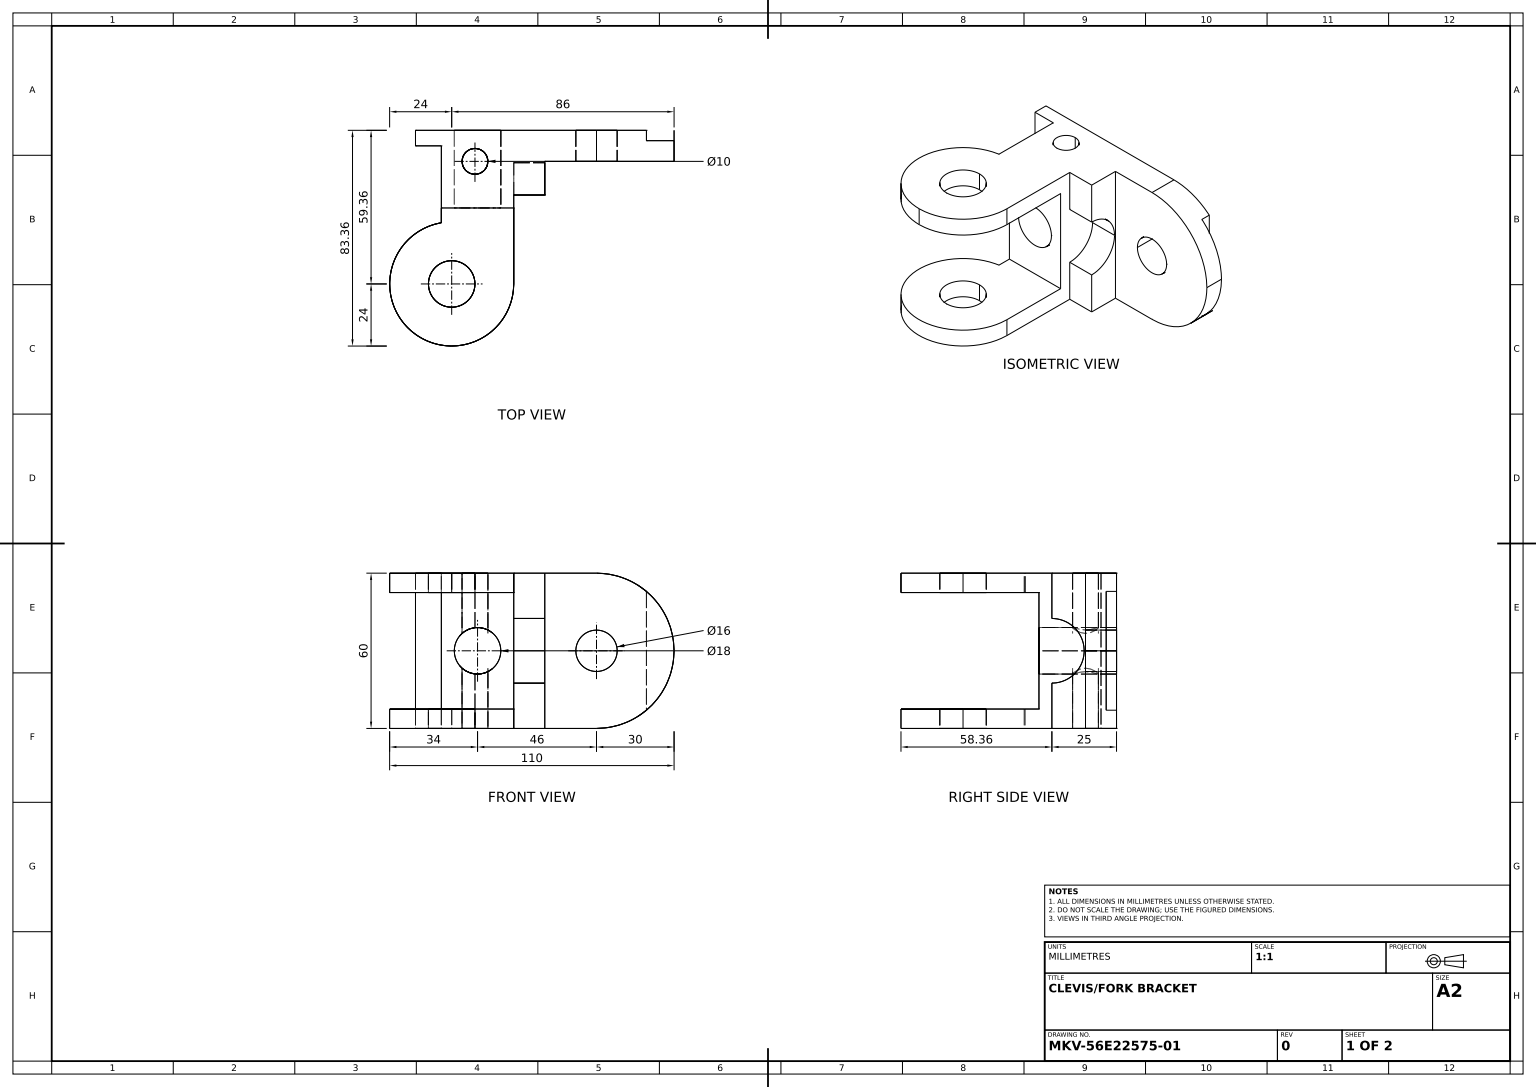
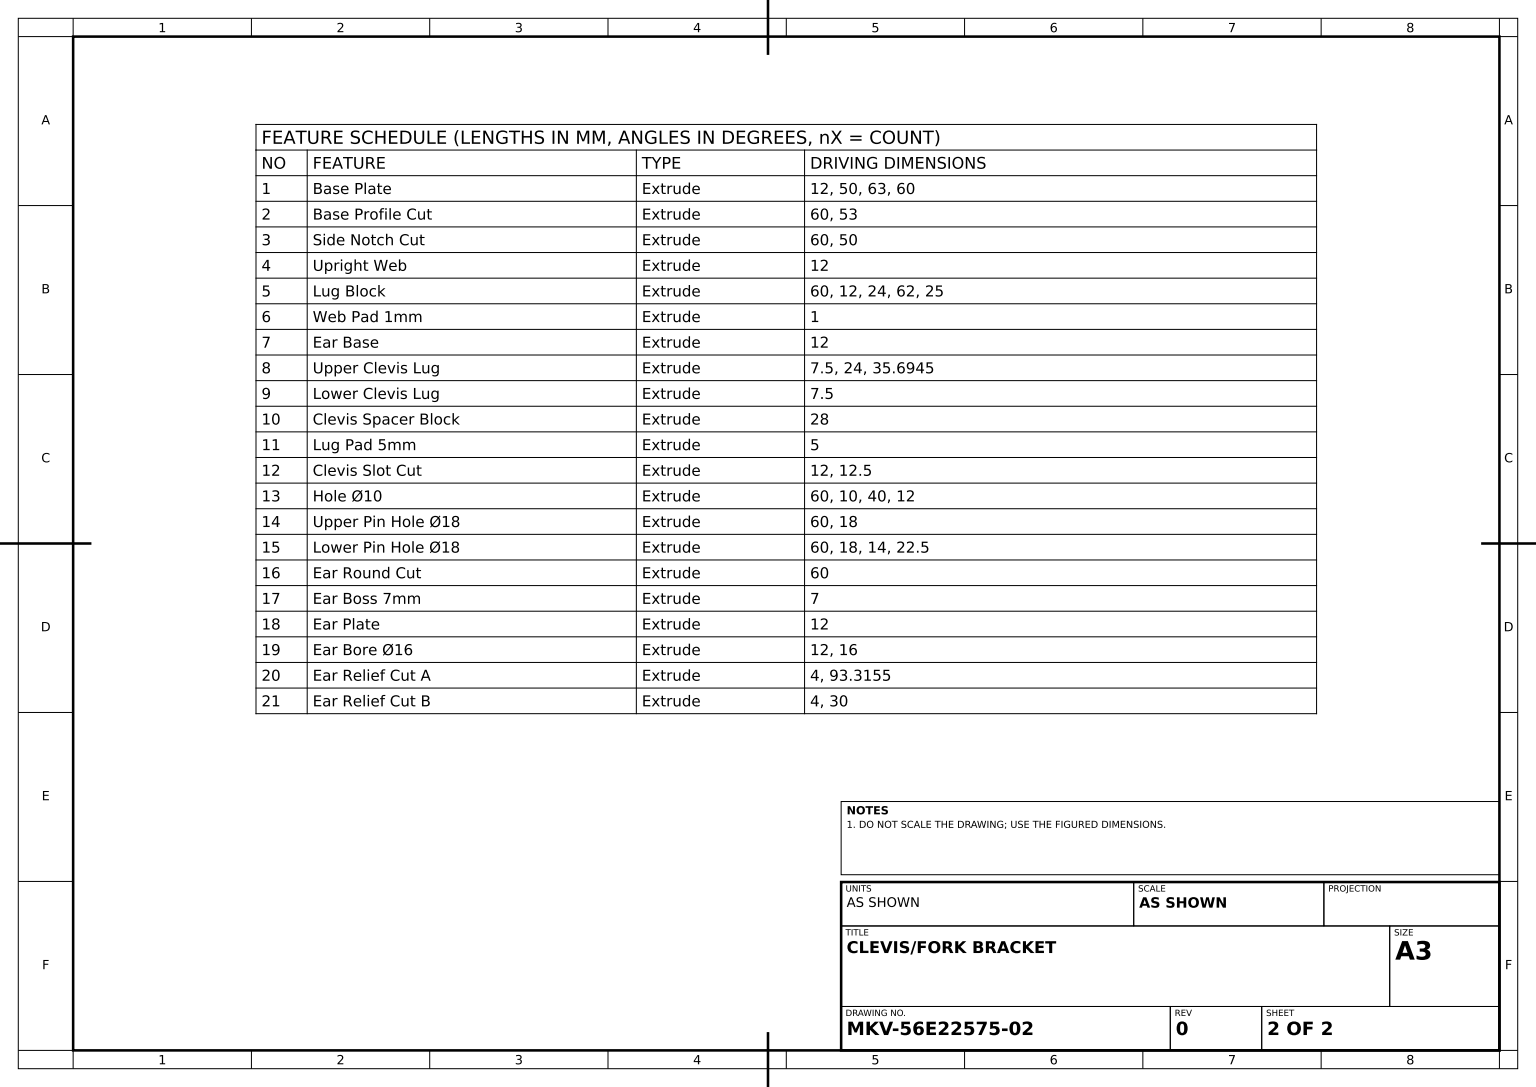
from build123d import *

# Parameters (mm, degrees)
BASE_PLATE_DEPTH           = 12
BASE_PROFILE_CUT_SKETCH_W  = 10
BASE_PROFILE_CUT_SKETCH_H  = 6
BASE_PROFILE_CUT_DEPTH     = 60
SIDE_NOTCH_SKETCH_W        = 13
SIDE_NOTCH_SKETCH_H        = 12
SIDE_NOTCH_CUT_DEPTH       = 60
UPRIGHT_WEB_SKETCH_W       = 12
UPRIGHT_WEB_SKETCH_H       = 60
UPRIGHT_WEB_DEPTH          = 12
LUG_BLOCK_SKETCH_W         = 12
LUG_BLOCK_SKETCH_H         = 13
LUG_BLOCK_DEPTH            = 60
WEB_PAD_SKETCH_W           = 12
WEB_PAD_SKETCH_H           = 60
WEB_PAD_1MM_DEPTH          = 1
EAR_BASE_DEPTH             = 12
UPPER_CLEVIS_LUG_DEPTH     = 7.5
LOWER_START                = -7.5
LOWER_CLEVIS_LUG_DEPTH     = 7.5
CLEVIS_SPACER_SKETCH_W     = 13
CLEVIS_SPACER_SKETCH_H     = 45
CLEVIS_SPACER_BLOCK_DEPTH  = 28
LUG_PAD_SKETCH_W           = 28
LUG_PAD_SKETCH_H           = 45
LUG_PAD_5MM_DEPTH          = 5
CLEVIS_SLOT_CUT_DEPTH      = 12
HOLE_10_SKETCH_R           = 5
HOLE_10_DEPTH              = 60
UPPER_PIN_HOLE_18_SKETCH_R = 9
UPPER_PIN_HOLE_18_DEPTH    = 60
LOWER_PIN_HOLE_18_SKETCH_R = 9
LOWER_PIN_HOLE_18_DEPTH    = 60
EAR_ROUND_CUT_DEPTH        = 60
EAR_BOSS_SKETCH_W          = 12
EAR_BOSS_SKETCH_H          = 60
EAR_BOSS_7MM_DEPTH         = 7
EAR_PLATE_DEPTH            = 12
EAR_BORE_16_SKETCH_R       = 8
EAR_BORE_16_DEPTH          = 12
EAR_START                  = -4
EAR_RELIEF_CUT_A_DEPTH     = 4
EAR_RELIEF_CUT_B_DEPTH     = 4


with BuildPart() as part:
    # Base Plate Sketch → Base Plate (new body)
    with BuildSketch(Plane.XY):
        Polygon((0, 0), (50, 0), (63, 0), (63, 60), (50, 60), (0, 60), align=None)
    extrude(amount=BASE_PLATE_DEPTH)

    # Base Profile Cut Sketch → Base Profile Cut (cut)
    with BuildSketch(Plane.XZ):
        with Locations((5, 9)):
            Rectangle(BASE_PROFILE_CUT_SKETCH_W, BASE_PROFILE_CUT_SKETCH_H)
    extrude(amount=-BASE_PROFILE_CUT_DEPTH, mode=Mode.SUBTRACT)

    # Side Notch Sketch → Side Notch Cut (cut)
    with BuildSketch(Plane.XZ):
        with Locations((56.5, 6)):
            Rectangle(SIDE_NOTCH_SKETCH_W, SIDE_NOTCH_SKETCH_H)
    extrude(amount=-SIDE_NOTCH_CUT_DEPTH, mode=Mode.SUBTRACT)

    # Upright Web Sketch → Upright Web (add)
    with BuildSketch(Plane.XY.offset(12)):
        with Locations((56, 30)):
            Rectangle(UPRIGHT_WEB_SKETCH_W, UPRIGHT_WEB_SKETCH_H)
    extrude(amount=-UPRIGHT_WEB_DEPTH)

    # Lug Block Sketch → Lug Block (add)
    with BuildSketch(Plane.XZ):
        with Locations((44, 18.5)):
            Rectangle(LUG_BLOCK_SKETCH_W, LUG_BLOCK_SKETCH_H)
    extrude(amount=-LUG_BLOCK_DEPTH)

    # Web Pad Sketch → Web Pad 1mm (add)
    with BuildSketch(Plane(origin=(62, 0, 0), x_dir=(0, 0, -1), z_dir=(1, 0, 0))):
        with Locations((-6, 30)):
            Rectangle(WEB_PAD_SKETCH_W, WEB_PAD_SKETCH_H)
    extrude(amount=WEB_PAD_1MM_DEPTH)

    # Ear Base Sketch → Ear Base (add)
    with BuildSketch(Plane.XY.offset(12)):
        with BuildLine():
            Line((63, 60), (63, 0))
            ThreePointArc((63, 0), (93, 30), (63, 60))
        make_face()
    extrude(amount=-EAR_BASE_DEPTH)

    # Upper Clevis Lug Sketch → Upper Clevis Lug (add)
    with BuildSketch(Plane.XZ):
        with BuildLine():
            Line((38, 59.358797437), (38, 25))
            Line((38, 25), (38, 12))
            Line((38, 12), (10, 12))
            Line((10, 12), (10, 35.694478304))
            ThreePointArc((10, 35.694478304), (-1.491933385, 77.689100216), (38, 59.358797437))
        make_face()
    extrude(amount=-UPPER_CLEVIS_LUG_DEPTH)

    # Lower Clevis Lug Sketch → Lower Clevis Lug (add)
    with BuildSketch(Plane(origin=(0, 60, 0), x_dir=(1, 0, 0), z_dir=(0, 1, 0)).offset(LOWER_START)):
        with BuildLine():
            Line((38, -12), (38, -59.358797437))
            ThreePointArc((38, -59.358797437), (-1.491933385, -77.689100216), (10, -35.694478304))
            Line((10, -35.694478304), (10, -12))
            Line((10, -12), (38, -12))
        make_face()
    extrude(amount=LOWER_CLEVIS_LUG_DEPTH)

    # Clevis Spacer Sketch → Clevis Spacer Block (add)
    with BuildSketch(Plane.ZY.offset(-38)):
        with Locations((18.5, 30)):
            Rectangle(CLEVIS_SPACER_SKETCH_W, CLEVIS_SPACER_SKETCH_H)
    extrude(amount=CLEVIS_SPACER_BLOCK_DEPTH)

    # Lug Pad Sketch → Lug Pad 5mm (add)
    with BuildSketch(Plane.XY.offset(25)):
        with Locations((24, 30)):
            Rectangle(LUG_PAD_SKETCH_W, LUG_PAD_SKETCH_H)
    extrude(amount=LUG_PAD_5MM_DEPTH)

    # Clevis Slot Sketch → Clevis Slot Cut (cut)
    with BuildSketch(Plane(origin=(50, 0, 0), x_dir=(0, 0, -1), z_dir=(1, 0, 0))):
        with BuildLine():
            Line((-25, 42.5), (-25, 17.5))
            ThreePointArc((-25, 17.5), (-12.5, 30), (-25, 42.5))
        make_face()
    extrude(amount=-CLEVIS_SLOT_CUT_DEPTH, mode=Mode.SUBTRACT)

    # Hole Ø10 Sketch → Hole Ø10 (cut)
    with BuildSketch(Plane.XZ):
        with Locations(Location((23, 12, 0), (0, 0, 270))):
            Circle(HOLE_10_SKETCH_R)
    extrude(amount=-HOLE_10_DEPTH, mode=Mode.SUBTRACT)

    # Upper Pin Hole Ø18 Sketch → Upper Pin Hole Ø18 (cut)
    with BuildSketch(Plane.XZ):
        with Locations(Location((14, 59.358797437, 0), (0, 0, 270))):
            Circle(UPPER_PIN_HOLE_18_SKETCH_R)
    extrude(amount=-UPPER_PIN_HOLE_18_DEPTH, mode=Mode.SUBTRACT)

    # Lower Pin Hole Ø18 Sketch → Lower Pin Hole Ø18 (cut)
    with BuildSketch(Plane.XY.offset(30)):
        with Locations((24, 30)):
            Circle(LOWER_PIN_HOLE_18_SKETCH_R)
    extrude(amount=-LOWER_PIN_HOLE_18_DEPTH, mode=Mode.SUBTRACT)

    # Ear Round Cut Sketch → Ear Round Cut (cut)
    with BuildSketch(Plane.XY.offset(12)):
        with BuildLine():
            Line((63, 60), (63, 0))
            ThreePointArc((63, 0), (93, 30), (63, 60))
        make_face()
    extrude(amount=-EAR_ROUND_CUT_DEPTH, mode=Mode.SUBTRACT)

    # Ear Boss Sketch → Ear Boss 7mm (add)
    with BuildSketch(Plane(origin=(63, 0, 0), x_dir=(0, 0, -1), z_dir=(1, 0, 0))):
        with Locations((-6, 30)):
            Rectangle(EAR_BOSS_SKETCH_W, EAR_BOSS_SKETCH_H)
    extrude(amount=EAR_BOSS_7MM_DEPTH)

    # Ear Plate Sketch → Ear Plate (add)
    with BuildSketch(Plane.XY.offset(12)):
        with BuildLine():
            Line((70, 60), (70, 0))
            ThreePointArc((70, 0), (100, 30), (70, 60))
        make_face()
    extrude(amount=-EAR_PLATE_DEPTH)

    # Ear Bore Ø16 Sketch → Ear Bore Ø16 (cut)
    with BuildSketch(Plane.XY.offset(12)):
        with Locations((70, 30)):
            Circle(EAR_BORE_16_SKETCH_R)
    extrude(amount=-EAR_BORE_16_DEPTH, mode=Mode.SUBTRACT)

    # Ear Relief A Sketch → Ear Relief Cut A (cut)
    with BuildSketch(Plane(origin=(0, 0, 0), x_dir=(-1, 0, 0), z_dir=(0, 0, -1)).offset(EAR_START)):
        with BuildLine():
            Line((-93.315470525, 48.878263537), (-93.315470525, 11.121736463))
            ThreePointArc((-93.315470525, 11.121736463), (-100, 30), (-93.315470525, 48.878263537))
        make_face()
    extrude(amount=EAR_RELIEF_CUT_A_DEPTH, mode=Mode.SUBTRACT)

    # Ear Relief B Sketch → Ear Relief Cut B (cut)
    with BuildSketch(Plane(origin=(0, 0, 0), x_dir=(-1, 0, 0), z_dir=(0, 0, -1)).offset(EAR_START)):
        with BuildLine():
            Line((-89.315470525, 7.045423149), (-89.315470525, 30))
            Line((-89.315470525, 30), (-89.315470525, 52.954576851))
            ThreePointArc((-89.315470525, 52.954576851), (-91.41269171, 51.011821285), (-93.315470525, 48.878263537))
            Line((-93.315470525, 48.878263537), (-93.315470525, 11.121736463))
            ThreePointArc((-93.315470525, 11.121736463), (-91.41269171, 8.988178715), (-89.315470525, 7.045423149))
        make_face()
    extrude(amount=EAR_RELIEF_CUT_B_DEPTH, mode=Mode.SUBTRACT)


solid = part.part
